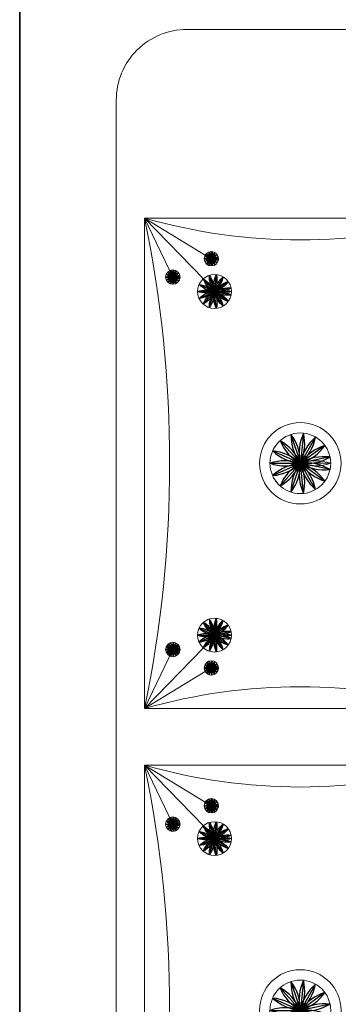
# Model space of a CAD drawing. Units: inches. Extents: x -61 to 1599, y -1316 to 257.
# Tile 175 of 204: x 1382 to 1395, y -684 to -643. Entities that reach past the tile are written whole.
import ezdxf

# ---------------------------------------------------------------- set-up
doc = ezdxf.new("R2010")
doc.units = ezdxf.units.IN
doc.header["$MEASUREMENT"] = 0
doc.layers.add('FURNITURE', color=83, linetype='Continuous', lineweight=18)
doc.layers.add('WALLS', color=4, linetype='Continuous', lineweight=35)
doc.layers.add('LT', color=8, linetype='Continuous')

# ---------------------------------------------------------------- blocks, each defined once
blk = doc.blocks.new('*U104')
at = {"layer": 'LT'}
blk.add_line((0, 0.152), (0, -0.152), dxfattribs=at)
for centre, start, end in [((0.443, 0), 160.9983, 199.0017), ((-0.443, 0), 340.9983, 19.0017)]:
    blk.add_arc(centre, 0.468, start, end, dxfattribs=at)
blk = doc.blocks.new('*U105')
at = {"layer": 'LT', "transparency": 16777216}
for p, rotation in [((-57.958, -16.311), 72), ((-57.926, -16.256), 48.00000000000001), ((-57.875, -16.219), 24), ((-57.751, -16.219), 336), ((-57.699, -16.256), 312), ((-57.668, -16.311), 288), ((-57.964, -16.374), 96), ((-57.945, -16.435), 120), ((-57.902, -16.482), 144), ((-57.844, -16.508), 168.0000000000001), ((-57.781, -16.508), 192), ((-57.723, -16.482), 216), ((-57.68, -16.435), 240), ((-57.661, -16.374), 264)]:
    blk.add_blockref('*U104', p, dxfattribs=dict(at, rotation=rotation))
blk.add_blockref('*U104', (-57.813, -16.206), dxfattribs=at)
blk = doc.blocks.new('*U71')
at = {"layer": 'LT'}
blk.add_line((0, 0.152), (0, -0.152), dxfattribs=at)
for centre, start, end in [((0.443, 0), 160.9983, 199.0017), ((-0.443, 0), 340.9983, 19.0017)]:
    blk.add_arc(centre, 0.468, start, end, dxfattribs=at)
blk = doc.blocks.new('*U58')
at = {"layer": 'LT', "transparency": 16777216}
for p, rotation in [((-57.958, -16.311), 72), ((-57.926, -16.256), 48.00000000000001), ((-57.875, -16.219), 24), ((-57.751, -16.219), 336), ((-57.699, -16.256), 312), ((-57.668, -16.311), 288), ((-57.964, -16.374), 96), ((-57.945, -16.435), 120), ((-57.902, -16.482), 144), ((-57.844, -16.508), 168.0000000000001), ((-57.781, -16.508), 192), ((-57.723, -16.482), 216), ((-57.68, -16.435), 240), ((-57.661, -16.374), 264)]:
    blk.add_blockref('*U71', p, dxfattribs=dict(at, rotation=rotation))
blk.add_blockref('*U71', (-57.813, -16.206), dxfattribs=at)
blk = doc.blocks.new('*U61')
at = {"layer": 'LT'}
blk.add_line((0, 0.152), (0, -0.152), dxfattribs=at)
for centre, start, end in [((0.443, 0), 160.9983, 199.0017), ((-0.443, 0), 340.9983, 19.0017)]:
    blk.add_arc(centre, 0.468, start, end, dxfattribs=at)
blk = doc.blocks.new('*U62')
at = {"layer": 'LT', "transparency": 16777216}
for p, rotation in [((-57.958, -16.311), 72), ((-57.926, -16.256), 48.00000000000001), ((-57.875, -16.219), 24), ((-57.751, -16.219), 336), ((-57.699, -16.256), 312), ((-57.668, -16.311), 288), ((-57.964, -16.374), 96), ((-57.945, -16.435), 120), ((-57.902, -16.482), 144), ((-57.844, -16.508), 168.0000000000001), ((-57.781, -16.508), 192), ((-57.723, -16.482), 216), ((-57.68, -16.435), 240), ((-57.661, -16.374), 264)]:
    blk.add_blockref('*U61', p, dxfattribs=dict(at, rotation=rotation))
blk.add_blockref('*U61', (-57.813, -16.206), dxfattribs=at)
blk = doc.blocks.new('*U57')
at = {"layer": 'LT'}
blk.add_line((0, 0.359), (0, -0.359), dxfattribs=at)
for centre, start, end in [((1.041, 0), 160.9983, 199.0017), ((-1.041, 0), 340.9983, 19.0017)]:
    blk.add_arc(centre, 1.101, start, end, dxfattribs=at)
blk = doc.blocks.new('*U99')
at = {"layer": 'LT', "transparency": 16777216}
for p, rotation in [((-136.227, -38.231), 48.00000000000001), ((-136.107, -38.143), 23.99999999999999), ((-135.815, -38.143), 336.0000000000001), ((-135.694, -38.231), 312), ((-136.318, -38.508), 96), ((-136.302, -38.36), 72), ((-135.62, -38.36), 288.0000000000001), ((-135.604, -38.508), 264), ((-136.271, -38.65), 120), ((-136.172, -38.761), 144), ((-136.035, -38.822), 168.0000000000001), ((-135.886, -38.822), 191.9999999999999), ((-135.75, -38.761), 216), ((-135.65, -38.65), 240)]:
    blk.add_blockref('*U57', p, dxfattribs=dict(at, rotation=rotation))
blk.add_blockref('*U57', (-135.961, -38.112), dxfattribs=at)
blk = doc.blocks.new('*U80')
at = {"layer": 'LT'}
blk.add_line((0, 0.359), (0, -0.359), dxfattribs=at)
for centre, start, end in [((1.041, 0), 160.9983, 199.0017), ((-1.041, 0), 340.9983, 19.0017)]:
    blk.add_arc(centre, 1.101, start, end, dxfattribs=at)
blk = doc.blocks.new('*U96')
at = {"layer": 'LT', "transparency": 16777216}
for p, rotation in [((-136.227, -38.231), 48.00000000000001), ((-136.107, -38.143), 23.99999999999999), ((-135.815, -38.143), 336.0000000000001), ((-135.694, -38.231), 312), ((-136.318, -38.508), 96), ((-136.302, -38.36), 72), ((-135.62, -38.36), 288.0000000000001), ((-135.604, -38.508), 264), ((-136.271, -38.65), 120), ((-136.172, -38.761), 144), ((-136.035, -38.822), 168.0000000000001), ((-135.886, -38.822), 191.9999999999999), ((-135.75, -38.761), 216), ((-135.65, -38.65), 240)]:
    blk.add_blockref('*U80', p, dxfattribs=dict(at, rotation=rotation))
blk.add_blockref('*U80', (-135.961, -38.112), dxfattribs=at)
blk = doc.blocks.new('*U69')
at = {"layer": 'LT'}
blk.add_line((0, 0.359), (0, -0.359), dxfattribs=at)
for centre, start, end in [((1.041, 0), 160.9983, 199.0017), ((-1.041, 0), 340.9983, 19.0017)]:
    blk.add_arc(centre, 1.101, start, end, dxfattribs=at)
blk = doc.blocks.new('*U70')
at = {"layer": 'LT', "transparency": 16777216}
for p, rotation in [((-136.227, -38.231), 48.00000000000001), ((-136.107, -38.143), 23.99999999999999), ((-135.815, -38.143), 336.0000000000001), ((-135.694, -38.231), 312), ((-136.318, -38.508), 96), ((-136.302, -38.36), 72), ((-135.62, -38.36), 288.0000000000001), ((-135.604, -38.508), 264), ((-136.271, -38.65), 120), ((-136.172, -38.761), 144), ((-136.035, -38.822), 168.0000000000001), ((-135.886, -38.822), 191.9999999999999), ((-135.75, -38.761), 216), ((-135.65, -38.65), 240)]:
    blk.add_blockref('*U69', p, dxfattribs=dict(at, rotation=rotation))
blk.add_blockref('*U69', (-135.961, -38.112), dxfattribs=at)
blk = doc.blocks.new('*U55')
at = {"layer": 'LT'}
blk.add_line((0, 0.152), (0, -0.152), dxfattribs=at)
for centre, start, end in [((0.443, 0), 160.9983, 199.0017), ((-0.443, 0), 340.9983, 19.0017)]:
    blk.add_arc(centre, 0.468, start, end, dxfattribs=at)
blk = doc.blocks.new('*U56')
at = {"layer": 'LT', "transparency": 16777216}
for p, rotation in [((-57.958, -16.311), 72), ((-57.926, -16.256), 48.00000000000001), ((-57.875, -16.219), 24), ((-57.751, -16.219), 336), ((-57.699, -16.256), 312), ((-57.668, -16.311), 288), ((-57.964, -16.374), 96), ((-57.945, -16.435), 120), ((-57.902, -16.482), 144), ((-57.844, -16.508), 168.0000000000001), ((-57.781, -16.508), 192), ((-57.723, -16.482), 216), ((-57.68, -16.435), 240), ((-57.661, -16.374), 264)]:
    blk.add_blockref('*U55', p, dxfattribs=dict(at, rotation=rotation))
blk.add_blockref('*U55', (-57.813, -16.206), dxfattribs=at)
blk = doc.blocks.new('*U59')
at = {"layer": 'LT'}
blk.add_line((0, 0.152), (0, -0.152), dxfattribs=at)
for centre, start, end in [((0.443, 0), 160.9983, 199.0017), ((-0.443, 0), 340.9983, 19.0017)]:
    blk.add_arc(centre, 0.468, start, end, dxfattribs=at)
blk = doc.blocks.new('*U60')
at = {"layer": 'LT', "transparency": 16777216}
for p, rotation in [((-57.958, -16.311), 72), ((-57.926, -16.256), 48.00000000000001), ((-57.875, -16.219), 24), ((-57.751, -16.219), 336), ((-57.699, -16.256), 312), ((-57.668, -16.311), 288), ((-57.964, -16.374), 96), ((-57.945, -16.435), 120), ((-57.902, -16.482), 144), ((-57.844, -16.508), 168.0000000000001), ((-57.781, -16.508), 192), ((-57.723, -16.482), 216), ((-57.68, -16.435), 240), ((-57.661, -16.374), 264)]:
    blk.add_blockref('*U59', p, dxfattribs=dict(at, rotation=rotation))
blk.add_blockref('*U59', (-57.813, -16.206), dxfattribs=at)
blk = doc.blocks.new('*U67')
at = {"layer": 'LT'}
blk.add_line((0, 0.152), (0, -0.152), dxfattribs=at)
for centre, start, end in [((0.443, 0), 160.9983, 199.0017), ((-0.443, 0), 340.9983, 19.0017)]:
    blk.add_arc(centre, 0.468, start, end, dxfattribs=at)
blk = doc.blocks.new('*U68')
at = {"layer": 'LT', "transparency": 16777216}
for p, rotation in [((-57.958, -16.311), 72), ((-57.926, -16.256), 48.00000000000001), ((-57.875, -16.219), 24), ((-57.751, -16.219), 336), ((-57.699, -16.256), 312), ((-57.668, -16.311), 288), ((-57.964, -16.374), 96), ((-57.945, -16.435), 120), ((-57.902, -16.482), 144), ((-57.844, -16.508), 168.0000000000001), ((-57.781, -16.508), 192), ((-57.723, -16.482), 216), ((-57.68, -16.435), 240), ((-57.661, -16.374), 264)]:
    blk.add_blockref('*U67', p, dxfattribs=dict(at, rotation=rotation))
blk.add_blockref('*U67', (-57.813, -16.206), dxfattribs=at)
blk = doc.blocks.new('*U106')
at = {"layer": 'LT'}
blk.add_line((0, 0.643), (0, -0.643), dxfattribs=at)
for centre, start, end in [((1.867, 0), 160.9983, 199.0017), ((-1.867, 0), 340.9983, 19.0017)]:
    blk.add_arc(centre, 1.975, start, end, dxfattribs=at)
blk = doc.blocks.new('*U93')
at = {"layer": 'LT', "transparency": 16777216}
for p, rotation in [((-244.201, -68.532), 48.00000000000001), ((-243.984, -68.375), 23.99999999999999), ((-243.461, -68.375), 336.0000000000001), ((-243.245, -68.532), 312), ((-244.334, -68.764), 72), ((-243.111, -68.764), 288), ((-244.362, -69.03), 96), ((-244.28, -69.284), 120), ((-243.166, -69.284), 240), ((-243.083, -69.03), 264), ((-244.101, -69.483), 144), ((-243.856, -69.591), 168), ((-243.589, -69.591), 192), ((-243.345, -69.483), 216)]:
    blk.add_blockref('*U106', p, dxfattribs=dict(at, rotation=rotation))
blk.add_blockref('*U106', (-243.723, -68.32), dxfattribs=at)
blk = doc.blocks.new('*U63')
at = {"layer": 'LT'}
blk.add_line((0, 0.643), (0, -0.643), dxfattribs=at)
for centre, start, end in [((1.867, 0), 160.9983, 199.0017), ((-1.867, 0), 340.9983, 19.0017)]:
    blk.add_arc(centre, 1.975, start, end, dxfattribs=at)
blk = doc.blocks.new('*U64')
at = {"layer": 'LT', "transparency": 16777216}
for p, rotation in [((-244.201, -68.532), 48.00000000000001), ((-243.984, -68.375), 23.99999999999999), ((-243.461, -68.375), 336.0000000000001), ((-243.245, -68.532), 312), ((-244.334, -68.764), 72), ((-243.111, -68.764), 288), ((-244.362, -69.03), 96), ((-244.28, -69.284), 120), ((-243.166, -69.284), 240), ((-243.083, -69.03), 264), ((-244.101, -69.483), 144), ((-243.856, -69.591), 168), ((-243.589, -69.591), 192), ((-243.345, -69.483), 216)]:
    blk.add_blockref('*U63', p, dxfattribs=dict(at, rotation=rotation))
blk.add_blockref('*U63', (-243.723, -68.32), dxfattribs=at)
blk = doc.blocks.new('BED-DOUBLE-COMPACT')
for p, q in [((1.2, 52.036), (14.4, 52.036)), ((1.2, 52.036), (2.398, 49.532)), ((1.2, 52.036), (4.201, 48.934)), ((1.2, 52.036), (4.028, 50.312)), ((4.028, 50.312), (4.333, 50.312)), ((2.398, 49.532), (2.703, 49.532)), ((4.165, 48.922), (4.882, 48.922)), ((7.8, 41.636), (9.086, 41.636)), ((1.2, 31.236), (4.201, 34.339)), ((4.165, 34.351), (4.882, 34.351)), ((1.2, 31.236), (2.398, 33.74)), ((2.398, 33.74), (2.703, 33.74)), ((1.2, 31.236), (4.028, 32.961)), ((4.028, 32.961), (4.333, 32.961)), ((1.2, 31.236), (1.2, 31.236)), ((1.2, 28.836), (14.4, 28.836)), ((1.2, 28.836), (2.398, 26.332)), ((1.2, 28.836), (4.201, 25.734)), ((1.2, 28.836), (4.028, 27.112)), ((4.028, 27.112), (4.333, 27.112)), ((2.398, 26.332), (2.703, 26.332)), ((4.165, 25.722), (4.882, 25.722))]:
    blk.add_line(p, q)
for points in [[(77, 60.036), (3, 60.036, 0.414214), (0, 57.036), (0, 3.036, 0.414214), (3, 0.036), (77, 0.036, 0.414214), (80, 3.036), (80, 57.036, 0.414214)], [(4.333, 50.312, 0.167358), (4.028, 50.312, 0.167358)], [(2.703, 49.532, 0.167358), (2.398, 49.532, 0.167358)], [(4.882, 48.922, 0.167358), (4.165, 48.922, 0.167358)], [(7.8, 41.636, 0.167358), (9.086, 41.636, 0.167358)], [(4.165, 34.351, 0.167358), (4.882, 34.351, 0.167358)], [(2.398, 33.74, 0.167358), (2.703, 33.74, 0.167358)], [(4.028, 32.961, 0.167358), (4.333, 32.961, 0.167358)], [(4.333, 27.112, 0.167358), (4.028, 27.112, 0.167358)], [(2.703, 26.332, 0.167358), (2.398, 26.332, 0.167358)], [(4.882, 25.722, 0.167358), (4.165, 25.722, 0.167358)]]:
    blk.add_lwpolyline(points, format="xyb", close=True)
for points in [[(14.4, 31.236), (1.2, 31.236), (1.2, 52.036), (14.4, 52.036), (14.4, 31.236), (1.2, 31.236), (1.2, 52.036)], [(14.4, 8.036), (1.2, 8.036), (1.2, 28.836)]]:
    blk.add_lwpolyline(points)
for centre, radius in [((4.028, 50.312), 0.305), ((2.398, 49.532), 0.305), ((4.165, 48.922), 0.717), ((7.8, 41.636), 1.724), ((7.8, 41.636), 1.286), ((4.165, 34.351), 0.717), ((2.398, 33.74), 0.305), ((4.028, 32.961), 0.305), ((4.028, 27.112), 0.305), ((2.398, 26.332), 0.305), ((4.165, 25.722), 0.717), ((7.8, 18.436), 1.724), ((7.8, 18.436), 1.286)]:
    blk.add_circle(centre, radius)
for centre, radius, start, end in [((-49.227, 41.636), 51.488, 348.3468, 11.6532), ((7.8, 75.06), 23.951, 254.0046, 285.9954), ((7.8, 8.212), 23.951, 74.0046, 105.9954), ((-49.227, 18.436), 51.488, 348.3468, 11.6532), ((7.8, 51.86), 23.951, 254.0046, 285.9954)]:
    blk.add_arc(centre, radius, start, end)
at = {"xscale": -1, "rotation": 90}
for name, p in [('*U68', (-12.33, -7.501)), ('*U62', (-13.96, -8.28)), ('*U70', (-34.306, -87.039)), ('*U56', (-12.33, -30.701)), ('*U105', (-13.96, -31.48)), ('*U99', (-34.306, -110.239))]:
    blk.add_blockref(name, p, dxfattribs=at)
at = {"rotation": 89.99999999999999}
for name, p in [('*U64', (-61.162, 285.359)), ('*U96', (-34.306, 170.312)), ('*U58', (-13.96, 91.553)), ('*U60', (-12.33, 90.773)), ('*U93', (-61.162, 262.159))]:
    blk.add_blockref(name, p, dxfattribs=at)

msp = doc.modelspace()

# ---------------------------------------------------------------- linework, layer by layer
at = {"layer": 'WALLS'}
msp.add_line((1381.7028, -621.169), (1381.7028, -729.169), dxfattribs=at)

# ---------------------------------------------------------------- block references
at = {"layer": 'FURNITURE'}
msp.add_blockref('BED-DOUBLE-COMPACT', (1385.794, -703.1131), dxfattribs=at)

doc.saveas('drawing.dxf')
